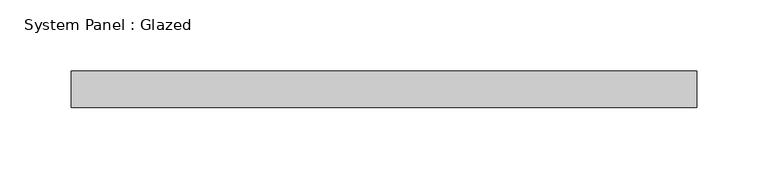
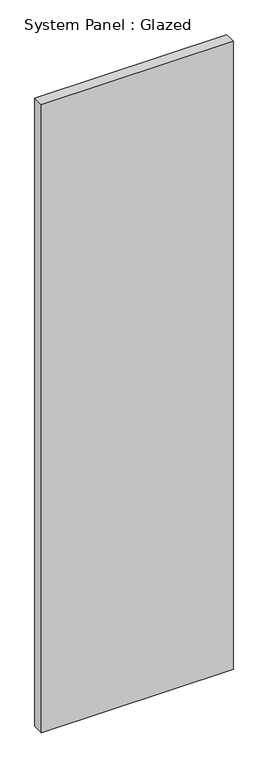
"""IFC4 building model written with IfcOpenShell, lengths in millimetres: plate geometry, System Panel : Glazed."""

from ifc_helpers import new_model, si_unit, origin, origin_with_axes, place, context, project, spatial, polyline, outline, extrude, source, transform, mapped, element, save


def system_panel_glazed_673a7a74(model_context):
    return source(origin(), model_context, "Body", "SweptSolid", [
        extrude(outline(polyline([(219.075, 19.05), (-219.075, 19.05), (-219.075, 44.45), (219.075, 44.45), (219.075, 19.05)])), origin_with_axes(), (0.0, 0.0, 1.0), 1517.7338557),
    ])


if __name__ == "__main__":
    model = new_model("IFC4")
    model_context = context("Model", 3, world=origin())
    ifc_project = project(units=[si_unit("LENGTHUNIT", "METRE", prefix="MILLI")], contexts=[model_context])
    site = spatial("IfcSite", under=ifc_project)
    building = spatial("IfcBuilding", under=site)
    placement = place(None, origin())
    system_panel_glazed_shape = system_panel_glazed_673a7a74(model_context)
    element("IfcPlate", 1, ObjectType="System Panel : Glazed", at=placement, inside=building, context=model_context, shape_type="MappedRepresentation", body=[
        mapped(system_panel_glazed_shape, transform((0.0, 0.0, 0.0), x_axis=(1.0, 0.0, 0.0), y_axis=(0.0, 1.0, 0.0), z_axis=(0.0, 0.0, 1.0))),
    ])
    save(model, "model.ifc")

# Revit data of these elements
# Type "System Panel : Glazed"
#   Construction Type Id = "GSP4R"
#   Analytic Construction = "1/8 in Pilkington single glazing"
#   Visual Light Transmittance = 0.9
#   Solar Heat Gain Coefficient = 0.86
#   Heat Transfer Coefficient (U) = 1.18115 BTU/(h·ft²·°F)
#   Define Thermal Properties by = 1
# Element 1 (IfcPlate, "System Panel : Glazed")
#   Materials on its faces: "Glass"
# Materials
#   "Glass": class "Glass", colour RGB 0 128 192, transparency 0.75, Description = "Soda Lime Glass", Cost = 0
